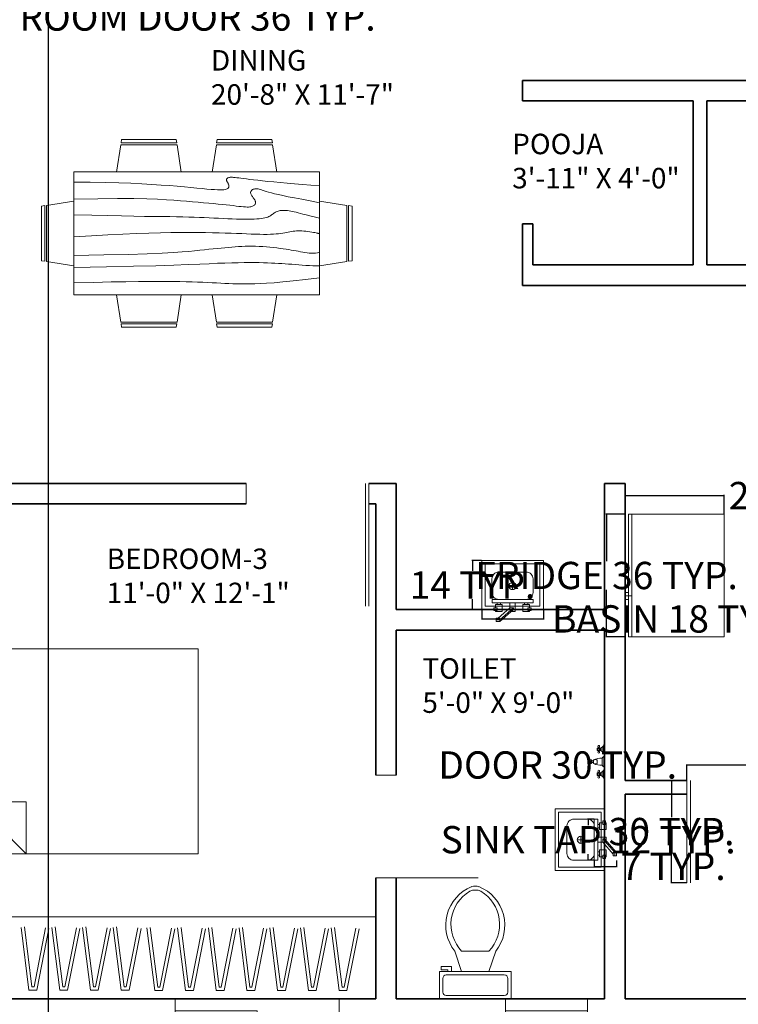
# Model space of a CAD drawing. Units: inches. Extents: x 3343 to 4790, y 1140 to 2641.
# Tile 4 of 10: x 3671 to 3881, y 2022 to 2310. Entities that reach past the tile are written whole.
import ezdxf

# ---------------------------------------------------------------- set-up
doc = ezdxf.new("R2010")
doc.units = ezdxf.units.IN
doc.header["$LTSCALE"] = 5
doc.header["$MEASUREMENT"] = 0
for name, color, linetype, lineweight in [('A-ANNO-DIMS', 2, 'Continuous', 18), ('A-AREA-IDEN', 7, 'Continuous', 18), ('A-DOOR', 3, 'Continuous', 18), ('A-EQPM', 9, 'Continuous', 18), ('A-FLOR-CASE', 9, 'Continuous', 18), ('A-FLOR-FIXT', 9, 'Continuous', 18), ('A-FURN', 8, 'Continuous', 13), ('A-GLAZ', 4, 'Continuous', 18), ('A-WALL', 7, 'Continuous', 35)]:
    doc.layers.add(name, color=color, linetype=linetype, lineweight=lineweight)
doc.styles.get("Standard").update_dxf_attribs({"font": 'arial.ttf'})
doc.dimstyles.get("Standard").update_dxf_attribs({"dimtxt": 8, "dimasz": 0.18, "dimexe": 0.18, "dimexo": 0.0625, "dimgap": 0.09, "dimtad": 0, "dimtih": 1, "dimtoh": 1, "dimdec": 1, "dimzin": 0, "dimdsep": 46, "dimlunit": 3, "dimtxsty": 'Standard', "dimcen": 0.09, "dimadec": 0, "dimazin": 0, "dimtfac": 1, "dimtdec": 1, "dimtofl": 0, "dimtmove": 0, "dimatfit": 3, "dimfxl": 1, "dimtolj": 1, "dimtzin": 0, "dimarcsym": 0})

# ---------------------------------------------------------------- blocks, each defined once
blk = doc.blocks.new('Bed - Queen')
for p, q in [((0, -80.00003), (0, 0)), ((0, 0), (59.99999, 0)), ((59.99999, 0), (59.99999, -80.00003)), ((7.99999, -1.2), (28.79998, -1.2)), ((7.99999, -14.4), (7.99999, -1.2)), ((28.79998, -1.2), (28.79998, -14.4)), ((31.19999, -1.2), (51.99999, -1.2)), ((31.19999, -14.4), (31.19999, -1.2)), ((51.99999, -1.2), (51.99999, -16.4)), ((0, -14.4), (44.8, -14.4)), ((59.99999, -29.6), (44.8, -14.4)), ((44.8, -14.4), (44.8, -29.6)), ((44.8, -16.8), (0, -16.8)), ((51.99999, -16.4), (46.79936, -16.4)), ((44.8, -29.6), (59.99999, -29.6)), ((59.99999, -80.00003), (0, -80.00003))]:
    blk.add_line(p, q)
blk = doc.blocks.new('Toilet - top')
for p, q in [((9.5, -6), (9.5, -2)), ((-10, -8.5), (-8, -8.5)), ((-10, -9.5), (-10, -8.5)), ((-8, -8.5), (-8, -8)), ((-7, -8), (-7, -9.5)), ((-4, -8), (-6, -14)), ((4, -8), (6, -14)), ((-7, -9.5), (-10, -9.5)), ((4, -14), (-4, -14))]:
    blk.add_line(p, q)
blk.add_lwpolyline([(10.5, -8), (10.5, 0), (-10.5, 0), (-10.5, -8)], close=True)
for points in [[(-9.5, -2), (-9.5, -6)], [(8.5, -1), (-8.5, -1)], [(-8.5, -7), (8.5, -7)]]:
    blk.add_lwpolyline(points)
for centre, radius, start, end in [((-8.62, -1.88), 0.884, 81.8699, 188.1301), ((8.62, -1.88), 0.884, 351.8699, 98.1301), ((-8.62, -6.12), 0.884, 171.8699, 278.1301), ((8.62, -6.12), 0.884, 261.8699, 8.1301), ((3.52, -21.58), 12.17, 141.4691, 247.9714), ((4.2, -21.82), 11.33, 136.3677, 238.9468), ((-3.52, -21.58), 12.17, 292.0284, 38.5307), ((-4.2, -21.82), 11.33, 301.053, 43.6321), ((0, -27.88), 4, 245.7318, 294.2682), ((0, -29), 4, 254.8605, 285.1395)]:
    blk.add_arc(centre, radius, start, end)
blk = doc.blocks.new('Faucet - Bathroom front')
for p, q in [((-0.5, 4.25), (0.5, 4.25)), ((0.5, 3.75), (-0.5, 3.75)), ((-0.5, 3), (0.5, 3)), ((-0.25, 3), (-0.25, 3.5)), ((0.25, 3.5), (0.25, 3)), ((-5, 0), (-2.25, 0)), ((-4.5087, 0.25), (-2.7408, 0.25)), ((-4, 1.625), (-4.25, 1.625)), ((-4, 1.375), (-4.25, 1.375)), ((-3.1442, 0.75), (-4.0979, 0.75)), ((-3.25, 1.625), (-3, 1.625)), ((-3.25, 1.375), (-3, 1.375)), ((-1.5, 0), (1.5, 0)), ((-1, 0.5), (1, 0.5)), ((0.5, 2), (-0.5, 2)), ((2.25, 0), (5, 0)), ((2.7413, 0.25), (4.5092, 0.25)), ((3.25, 1.625), (3, 1.625)), ((3.25, 1.375), (3, 1.375)), ((4.1058, 0.75), (3.1521, 0.75)), ((4, 1.625), (4.25, 1.625)), ((4, 1.375), (4.25, 1.375))]:
    blk.add_line(p, q)
for points in [[(-0.5, 3.75), (-0.5, 4.25)], [(-0.25, 4.5), (0.25, 4.5)], [(0.25, 3.5), (-0.25, 3.5)], [(0.5, 4.25), (0.5, 3.75)]]:
    blk.add_lwpolyline(points)
for points in [[(-4, 1), (-4, 2), (-3.25, 2), (-3.25, 1)], [(3.25, 1), (3.25, 2), (4, 2), (4, 1)]]:
    blk.add_lwpolyline(points, close=True)
for centre in [(-4.5, 1.5), (-3.625, 1.5), (-2.75, 1.5), (2.75, 1.5), (3.625, 1.5), (4.5, 1.5)]:
    blk.add_circle(centre, 0.2795)
for centre, radius, start, end in [((3, 1), 4.0311, 150.2551, 187.125), ((0.6413, 2.5), 1.246, 156.3417, 203.6583), ((-0.2575, 4.2575), 0.2426, 88.22243, 181.7776), ((-0.2575, 3.7425), 0.2426, 178.2224, 271.7776), ((0.2575, 4.2575), 0.2426, 358.2224, 91.77757), ((0.2575, 3.7425), 0.2426, 268.2224, 1.777565), ((-3, 1), 4.0311, 352.875, 29.74488), ((-0.6413, 2.5), 1.246, 336.3417, 23.65835), ((-5.375, 1.375), 1.4252, 285.2551, 344.7449), ((-1.875, 1.375), 1.4252, 195.2551, 254.7449), ((-0.7962, -0.2038), 0.7327, 106.1502, 163.8498), ((0.7962, -0.2038), 0.7327, 16.1502, 73.84979), ((1.875, 1.375), 1.4252, 285.2551, 344.7449), ((5.375, 1.375), 1.4252, 195.2551, 254.7449)]:
    blk.add_arc(centre, radius, start, end)
blk = doc.blocks.new('Faucet - kit sink front')
for p, q in [((-0.25, 3), (3.75, 6.5)), ((3.75, 6), (-0.25, 2.5)), ((3.75, 6), (3.75, 6.5)), ((3.75, 6.5), (4.75, 6.5)), ((3.75, 5.5), (3.75, 6)), ((4.75, 6), (3.75, 6)), ((4.75, 6.5), (4.75, 6)), ((4.75, 6), (4.75, 5.5)), ((-0.75, 3.5), (0.3192, 3.5)), ((-0.75, 1), (-0.75, 3.5)), ((-0.25, 2.5), (-0.25, 3)), ((4.1921, 5.5041), (0.75, 2.5)), ((4.75, 5.5), (3.75, 5.5)), ((-4.5, 1), (-4.5, 1.5)), ((-3.5, 1.5), (-3.5, 1)), ((0.75, 2.5), (-0.25, 2.5)), ((0.75, 2.5), (0.75, 1)), ((3.5, 1.5), (3.5, 1)), ((4.5, 1), (4.5, 1.5))]:
    blk.add_line(p, q)
for points in [[(-5.5, 2.5), (-5.5, 3.25), (-4.5, 3.25), (-4.5, 2.5)], [(5.5, 2.5), (5.5, 3.25), (4.5, 3.25), (4.5, 2.5)], [(-6, 0), (-6, 1), (6, 1), (6, 0)]]:
    blk.add_lwpolyline(points, close=True)
for points in [[(-5, 3.2513), (-5, 3.5), (-3, 3.5), (-3, 1.5), (-5, 1.5), (-5, 2.5)], [(5, 3.2513), (5, 3.5), (3, 3.5), (3, 1.5), (5, 1.5), (5, 2.5)]]:
    blk.add_lwpolyline(points)
blk = doc.blocks.new('Dining Set - 36 x 72 in.')
for p, q in [((-22.2343, 26.00059), (-23.4847, 17.99762)), ((-22.2304, 26), (-5.7608, 26)), ((-22, 27.5), (-22.1562, 26.50042)), ((-5.8416, 26.5), (-22.1534, 26.5)), ((-22, 27.5), (-6, 27.5)), ((-5.8437, 26.49966), (-6, 27.5)), ((-4.5152, 17.99762), (-5.7655, 25.99926)), ((5.7657, 26.00059), (4.5153, 17.99762)), ((5.7696, 26), (22.2392, 26)), ((6, 27.5), (5.8438, 26.50042)), ((22.1584, 26.5), (5.8466, 26.5)), ((6, 27.5), (22, 27.5)), ((22.1563, 26.49966), (22, 27.5)), ((23.4848, 17.99762), (22.2345, 25.99926)), ((36, 18), (-36, 18)), ((-36, 18), (-36, -18)), ((36, -18), (36, 18)), ((-44.0006, 8.23428), (-35.9976, 9.48474)), ((44.0006, 8.23428), (35.9976, 9.48474)), ((-45.5, 8), (-44.5004, 8.15617)), ((-45.5, 8), (-45.5, -8)), ((-44.5, -8.15843), (-44.5, 8.15338)), ((-44, 8.23041), (-44, -8.23915)), ((44, 8.23041), (44, -8.23915)), ((44.5, -8.15843), (44.5, 8.15338)), ((45.5, 8), (44.5005, 8.15617)), ((45.5, 8), (45.5, -8)), ((-44.4997, -8.15631), (-45.5, -8)), ((-35.9976, -9.48476), (-43.9993, -8.2345)), ((35.9976, -9.48476), (43.9993, -8.2345)), ((44.4997, -8.15631), (45.5, -8)), ((-36, -18), (36, -18)), ((-22.2343, -26.0006), (-23.4847, -17.99762)), ((-4.5152, -17.99762), (-5.7655, -25.99928)), ((5.7657, -26.0006), (4.5153, -17.99762)), ((23.4848, -17.99762), (22.2345, -25.99928)), ((-22.2304, -26), (-5.7608, -26)), ((-22, -27.5), (-22.1562, -26.50044)), ((-5.8416, -26.5), (-22.1534, -26.5)), ((-22, -27.5), (-6, -27.5)), ((-5.8437, -26.49967), (-6, -27.5)), ((5.7696, -26), (22.2392, -26)), ((6, -27.5), (5.8438, -26.50044)), ((22.1584, -26.5), (5.8466, -26.5)), ((6, -27.5), (22, -27.5)), ((22.1563, -26.49967), (22, -27.5))]:
    blk.add_line(p, q)
for points in [[(-36, 15), (-31.1772, 14.97754), (-26.8079, 14.91406), (-22.8538, 14.81543), (-19.276, 14.6875), (-16.0362, 14.53613), (-13.0957, 14.36718), (-10.4159, 14.18652), (-7.9583, 14), (-5.6904, 13.81315), (-3.6035, 13.63021), (-1.6954, 13.45508), (0.0365, 13.29166), (1.5945, 13.14388), (2.9811, 13.01562), (4.1988, 12.9108), (5.25, 12.83333), (6.1393, 12.78613), (6.8802, 12.76823), (7.4883, 12.77767), (7.9792, 12.8125), (8.3685, 12.87077), (8.6719, 12.95052), (8.9049, 13.0498), (9.0833, 13.16666), (9.2205, 13.29899), (9.3216, 13.44401), (9.3895, 13.59879), (9.4271, 13.76041), (9.4373, 13.92594), (9.4232, 14.09245), (9.3875, 14.257), (9.3333, 14.41666), (9.2638, 14.56917), (9.1836, 14.71484), (9.0975, 14.85465), (9.0104, 14.98958), (8.9272, 15.1206), (8.8529, 15.2487), (8.7922, 15.37483), (8.75, 15.5), (8.7305, 15.62467), (8.7344, 15.74739), (8.7617, 15.86621), (8.8125, 15.97916), (8.8867, 16.08431), (8.9844, 16.17968), (9.1055, 16.26334), (9.25, 16.33333), (9.4189, 16.38802), (9.6172, 16.42708), (9.8506, 16.45052), (10.125, 16.45833), (10.4463, 16.45052), (10.8203, 16.42708), (11.2529, 16.38802), (11.75, 16.33333), (12.3184, 16.26318), (12.9694, 16.17838), (13.7151, 16.07991), (14.5677, 15.96875), (15.5395, 15.84586), (16.6426, 15.71224), (17.8893, 15.56884), (19.2917, 15.41666), (20.859, 15.25667), (22.5879, 15.08984), (24.4721, 14.91715), (26.5052, 14.73958), (28.6809, 14.5581), (30.9929, 14.3737), (33.4347, 14.18733), (36, 14)], [(-36, 10), (-28.9766, 10.14274), (-23.1725, 10.20442), (-18.4241, 10.19775), (-14.5677, 10.13541), (-11.4399, 10.03011), (-8.877, 9.89453), (-6.7154, 9.74137), (-4.7917, 9.58333), (-2.9698, 9.43082), (-1.2246, 9.28515), (0.4415, 9.14534), (2.026, 9.01041), (3.5266, 8.87939), (4.9408, 8.7513), (6.266, 8.62516), (7.5, 8.5), (8.6411, 8.37549), (9.6914, 8.2539), (10.6538, 8.13818), (11.5312, 8.03125), (12.3267, 7.93603), (13.043, 7.85547), (13.6831, 7.79248), (14.25, 7.75), (14.7471, 7.7303), (15.1797, 7.73307), (15.5537, 7.75732), (15.875, 7.80208), (16.1494, 7.86637), (16.3828, 7.94922), (16.5811, 8.04964), (16.75, 8.16666), (16.8944, 8.29915), (17.0143, 8.44531), (17.1089, 8.60319), (17.1771, 8.77083), (17.218, 8.94629), (17.2305, 9.1276), (17.2137, 9.31282), (17.1667, 9.5), (17.0895, 9.6875), (16.987, 9.875), (16.8649, 10.0625), (16.7292, 10.25), (16.5856, 10.4375), (16.4401, 10.625), (16.2985, 10.8125), (16.1667, 11), (16.05, 11.18733), (15.9518, 11.3737), (15.8752, 11.5581), (15.8229, 11.73958), (15.798, 11.91715), (15.8034, 12.08984), (15.842, 12.25667), (15.9167, 12.41666), (16.0295, 12.56836), (16.1784, 12.70833), (16.3605, 12.83268), (16.5729, 12.9375), (16.8127, 13.01888), (17.0768, 13.07291), (17.3625, 13.0957), (17.6667, 13.08333), (17.9894, 13.03312), (18.3418, 12.94726), (18.7382, 12.82918), (19.1927, 12.68229), (19.7195, 12.51001), (20.3327, 12.31575), (21.0465, 12.10294), (21.875, 11.875), (22.8357, 11.63354), (23.959, 11.37304), (25.2786, 11.08618), (26.8282, 10.76562), (28.6414, 10.40405), (30.752, 9.99414), (33.1936, 9.52856), (36, 9)], [(-36, 5.5), (-30.7157, 5.3348), (-26.069, 5.20963), (-21.9946, 5.11767), (-18.4271, 5.05208), (-15.3009, 5.00602), (-12.5508, 4.97265), (-10.1112, 4.94515), (-7.9167, 4.91666), (-5.909, 4.88167), (-4.0586, 4.83984), (-2.3429, 4.79215), (-0.7396, 4.73958), (0.7739, 4.6831), (2.22, 4.6237), (3.6213, 4.56233), (5, 4.5), (6.373, 4.43782), (7.7344, 4.3776), (9.0723, 4.32129), (10.375, 4.27083), (11.6309, 4.22819), (12.8281, 4.19531), (13.9551, 4.17415), (15, 4.16666), (15.954, 4.17448), (16.819, 4.19791), (17.6001, 4.23698), (18.3021, 4.29166), (18.9299, 4.36198), (19.4883, 4.44791), (19.9823, 4.54948), (20.4167, 4.66666), (20.7969, 4.79899), (21.1302, 4.94401), (21.4245, 5.09879), (21.6875, 5.26041), (21.9271, 5.42594), (22.1511, 5.59245), (22.3672, 5.757), (22.5834, 5.91666), (22.8065, 6.06868), (23.0404, 6.21093), (23.2879, 6.34147), (23.5521, 6.45833), (23.8358, 6.55957), (24.142, 6.64323), (24.4735, 6.70735), (24.8334, 6.75), (25.2235, 6.76969), (25.642, 6.76692), (26.0858, 6.74267), (26.5521, 6.69791), (27.0379, 6.63362), (27.5404, 6.55078), (28.0565, 6.45036), (28.5834, 6.33333), (29.1242, 6.19987), (29.7071, 6.04687), (30.3661, 5.87044), (31.1354, 5.66666), (32.0493, 5.43164), (33.142, 5.16146), (34.4475, 4.85221), (36, 4.5)], [(-36, -1), (-30.7915, -0.6591), (-26.0195, -0.38216), (-21.6519, -0.16284), (-17.6563, 0.00521), (-14.0005, 0.12833), (-10.6523, 0.21289), (-7.5796, 0.26522), (-4.75, 0.29166), (-2.134, 0.29793), (0.2878, 0.28711), (2.5317, 0.26163), (4.6146, 0.22396), (6.5529, 0.17651), (8.3633, 0.12174), (10.0623, 0.06209), (11.6667, 0), (13.1899, -0.06201), (14.6341, -0.1211), (15.9982, -0.17432), (17.2813, -0.21875), (18.4823, -0.25147), (19.6003, -0.26953), (20.6343, -0.27002), (21.5834, -0.25), (22.4481, -0.20768), (23.2357, -0.14584), (23.9549, -0.06836), (24.6146, 0.02083), (25.2235, 0.11784), (25.7904, 0.21875), (26.3241, 0.31966), (26.8334, 0.41666), (27.3265, 0.50618), (27.8099, 0.58593), (28.2894, 0.65397), (28.7709, 0.70833), (29.2601, 0.74707), (29.763, 0.76823), (30.2855, 0.76985), (30.8334, 0.75), (31.4088, 0.70784), (31.9994, 0.64713), (32.589, 0.57275), (33.1615, 0.48958), (33.7008, 0.4025), (34.1908, 0.3164), (34.6153, 0.23616), (34.9584, 0.16666), (35.2099, 0.11165), (35.3848, 0.07031), (35.504, 0.04069), (35.5886, 0.02083), (35.6594, 0.00879), (35.7377, 0.0026), (35.8442, 0.00032), (36, 0)], [(-36, -6.5), (-27.1843, -6.31267), (-20.084, -6.1263), (-14.469, -5.9419), (-10.1094, -5.76042), (-6.7752, -5.58285), (-4.2363, -5.41016), (-2.2629, -5.24333), (-0.625, -5.08334), (0.8708, -4.93099), (2.2715, -4.78646), (3.5872, -4.64974), (4.8281, -4.52084), (6.0046, -4.39974), (7.127, -4.28646), (8.2053, -4.18099), (9.25, -4.08334), (10.2705, -3.99382), (11.2734, -3.91407), (12.2647, -3.84603), (13.25, -3.79167), (14.2354, -3.75293), (15.2266, -3.73177), (16.2295, -3.73015), (17.25, -3.75), (18.2912, -3.79248), (19.3451, -3.85547), (20.4009, -3.93604), (21.4479, -4.03125), (22.4754, -4.13819), (23.4727, -4.25391), (24.4289, -4.37549), (25.3334, -4.5), (26.1785, -4.62492), (26.9694, -4.74935), (27.7145, -4.87281), (28.4219, -4.99479), (29.1, -5.11483), (29.7572, -5.23242), (30.4016, -5.34709), (31.0417, -5.45834), (31.6837, -5.56437), (32.3262, -5.65821), (32.9658, -5.73153), (33.599, -5.77604), (34.2224, -5.78345), (34.8327, -5.74545), (35.4264, -5.65373), (36, -5.5)], [(-36, -10), (-26.4022, -9.81299), (-18.4675, -9.62891), (-11.9839, -9.45069), (-6.7396, -9.28125), (-2.5226, -9.12354), (0.8789, -8.98047), (3.6769, -8.85498), (6.0833, -8.75), (8.2767, -8.66765), (10.3021, -8.60677), (12.1712, -8.56543), (13.8958, -8.54167), (15.4876, -8.53353), (16.9583, -8.53907), (18.3197, -8.55632), (19.5834, -8.58334), (20.7616, -8.61841), (21.8685, -8.66081), (22.9188, -8.71004), (23.9271, -8.76563), (24.9081, -8.82707), (25.8763, -8.89388), (26.8465, -8.96558), (27.8334, -9.04167), (28.8474, -9.12118), (29.8828, -9.20117), (30.93, -9.27824), (31.9792, -9.34896), (33.0205, -9.40991), (34.0443, -9.45768), (35.0407, -9.48885), (36, -9.5)], [(-36, -14.5), (-30.0881, -14.33513), (-25.0332, -14.21224), (-20.7312, -14.12647), (-17.0781, -14.07292), (-13.97, -14.04671), (-11.3027, -14.04297), (-8.9724, -14.05681), (-6.875, -14.08334), (-4.9224, -14.11833), (-3.0905, -14.16016), (-1.3709, -14.20785), (0.2448, -14.26042), (1.7647, -14.3169), (3.1973, -14.3763), (4.5507, -14.43767), (5.8333, -14.5), (7.0554, -14.5621), (8.235, -14.62175), (9.3922, -14.67652), (10.5469, -14.72396), (11.7192, -14.76164), (12.929, -14.78711), (14.1965, -14.79794), (15.5417, -14.79167), (16.9933, -14.76424), (18.6152, -14.70508), (20.4804, -14.60197), (22.6615, -14.44271), (25.2312, -14.21509), (28.2624, -13.9069), (31.8277, -13.50594), (36, -13)]]:
    blk.add_lwpolyline(points)
blk = doc.blocks.new('Refrigerator-2 door - 36 in top')
for p, q in [((0, -26.999999), (36, -26.999999)), ((11, -27.999999), (11, -28.999999)), ((12, -26.999999), (12, -28.999999)), ((13, -28.999999), (13, -27.999999)), ((11, -28.999999), (13, -28.999999))]:
    blk.add_line(p, q)
blk.add_lwpolyline([(0, -27.999999), (0, 0), (36, 0), (36, -27.999999)], close=True)
blk = doc.blocks.new('SINK-BOWL-WITH-DRAIN')
for p, q in [((8.58, 9.03), (6.47, 9.03)), ((7.52, 10.09), (7.52, 7.97))]:
    blk.add_line(p, q)
for points in [[(14.44, 0), (0, 0), (0, 18.06), (14.44, 18.06)], [(1, 1), (1, 17.06), (13.44, 17.06), (13.44, 1)]]:
    blk.add_lwpolyline(points, close=True)
blk.add_lwpolyline([(9.44, 15.06), (5.44, 15.06, 0.414214), (3.44, 13.06), (3.44, 5, 0.414214), (5.44, 3), (9.44, 3, 0.414214), (11.44, 5), (11.44, 13.06, 0.414214)], format="xyb", close=True)
blk.add_circle((7.52, 9.03), 1.06)
blk = doc.blocks.new('WINDOW-48IN-SLIDING-JAMB9')
for p, q in [((0, 9), (0, 0)), ((48, 9), (48, 0)), ((0, 5.5), (24, 5.5)), ((0, 4.5), (48, 4.5)), ((24, 5.5), (24, 3.5)), ((24, 3.5), (48, 3.5))]:
    blk.add_line(p, q)
blk = doc.blocks.new('WINDOW-24IN-FIXED')
for p, q in [((0, 9), (0, 0)), ((24, 9), (24, 0)), ((0, 5.5), (24, 5.5)), ((0, 3.5), (24, 3.5))]:
    blk.add_line(p, q)
blk = doc.blocks.new('DOOR-36IN-6IN-JAMB-DBL-LINE')
at = {"ltscale": 5}
for p, q in [((35, 0), (35, 36)), ((36, 0), (36, 36)), ((0, 6), (0, 0)), ((36, 6), (36, 0))]:
    blk.add_line(p, q, dxfattribs=at)
blk = doc.blocks.new('DOOR-30IN-4IN-JAMB-DBL-LINE')
at = {"ltscale": 5}
for p, q in [((29, 0), (29, 30)), ((30, 0), (30, 30)), ((0, 4), (0, 0)), ((30, 4), (30, 0))]:
    blk.add_line(p, q, dxfattribs=at)
blk = doc.blocks.new('WARDROBE-HANGER')
for points in [[(0.22, 7.19), (17.51, 3.78), (17.51, 3.18), (0, 0.99)], [(0.41, 8.17), (18.51, 4.61), (18.51, 2.3), (0.12, 0)]]:
    blk.add_lwpolyline(points)
blk = doc.blocks.new('*D33')
at = {"layer": 'A-ANNO-DIMS', "color": 0, "lineweight": -2, "ltscale": 5, "transparency": 16777216}
for p, q in [((3839.07, 2075.77), (3837.15, 2075.77)), ((3837.33, 2075.59), (3837.33, 2073.99)), ((3837.33, 2063.95), (3837.33, 2065.54)), ((3839.07, 2063.77), (3837.15, 2063.77))]:
    blk.add_line(p, q, dxfattribs=at)
at = {"layer": 'A-ANNO-DIMS', "color": 0, "ltscale": 5, "transparency": 16777216}
for points in [[(3837.3, 2075.59), (3837.36, 2075.59), (3837.33, 2075.77)], [(3837.3, 2063.95), (3837.36, 2063.95), (3837.33, 2063.77)]]:
    blk.add_solid(points, dxfattribs=at)
at = {"layer": 'Defpoints', "color": 0, "ltscale": 5, "transparency": 16777216}
for p in [(3839.13, 2075.77), (3837.33, 2063.77), (3839.13, 2063.77)]:
    blk.add_point(p, dxfattribs=at)
at = {"layer": 'A-ANNO-DIMS', "color": 0, "ltscale": 5, "transparency": 16777216, "insert": (3837.33, 2069.77), "char_height": 8, "attachment_point": 5}
blk.add_mtext('\\A1;SINK TAP 12 TYP.', dxfattribs=at)
blk = doc.blocks.new('*D34')
at = {"layer": 'A-ANNO-DIMS', "color": 0, "lineweight": -2, "ltscale": 5, "transparency": 16777216}
for p, q in [((3839.13, 2063.7), (3839.13, 2061.79)), ((3845.63, 2063.7), (3845.63, 2061.79)), ((3839.31, 2061.97), (3845.45, 2061.97)), ((3845.63, 2061.97), (3845.81, 2061.97))]:
    blk.add_line(p, q, dxfattribs=at)
at = {"layer": 'A-ANNO-DIMS', "color": 0, "ltscale": 5, "transparency": 16777216}
for points in [[(3839.31, 2062), (3839.31, 2061.94), (3839.13, 2061.97)], [(3845.45, 2062), (3845.45, 2061.94), (3845.63, 2061.97)]]:
    blk.add_solid(points, dxfattribs=at)
at = {"layer": 'Defpoints', "color": 0, "ltscale": 5, "transparency": 16777216}
for p in [(3839.13, 2063.77), (3845.63, 2063.77), (3845.63, 2061.97)]:
    blk.add_point(p, dxfattribs=at)
at = {"layer": 'A-ANNO-DIMS', "color": 0, "ltscale": 5, "transparency": 16777216, "insert": (3862.23, 2061.97), "char_height": 8, "attachment_point": 5}
blk.add_mtext('\\A1;7 TYP.', dxfattribs=at)
blk = doc.blocks.new('*D51')
at = {"layer": 'A-ANNO-DIMS', "color": 0, "lineweight": -2, "ltscale": 5, "transparency": 16777216}
for p, q in [((3806.15, 2137.1), (3806.15, 2134.27)), ((3824.22, 2137.1), (3824.22, 2134.27)), ((3806.33, 2134.45), (3824.04, 2134.45)), ((3824.22, 2134.45), (3824.4, 2134.45))]:
    blk.add_line(p, q, dxfattribs=at)
at = {"layer": 'A-ANNO-DIMS', "color": 0, "ltscale": 5, "transparency": 16777216}
for points in [[(3806.33, 2134.48), (3806.33, 2134.42), (3806.15, 2134.45)], [(3824.04, 2134.48), (3824.04, 2134.42), (3824.22, 2134.45)]]:
    blk.add_solid(points, dxfattribs=at)
at = {"layer": 'Defpoints', "color": 0, "ltscale": 5, "transparency": 16777216}
for p in [(3806.15, 2137.16), (3824.22, 2137.16), (3824.22, 2134.45)]:
    blk.add_point(p, dxfattribs=at)
at = {"layer": 'A-ANNO-DIMS', "color": 0, "ltscale": 5, "transparency": 16777216, "insert": (3862.1, 2134.45), "char_height": 8, "attachment_point": 5}
blk.add_mtext('\\A1;BASIN 18 TYP.', dxfattribs=at)
blk = doc.blocks.new('*D52')
at = {"layer": 'A-ANNO-DIMS', "color": 0, "lineweight": -2, "ltscale": 5, "transparency": 16777216}
for p, q in [((3806.09, 2151.6), (3803.27, 2151.6)), ((3803.45, 2151.42), (3803.45, 2148.49)), ((3803.45, 2137.34), (3803.45, 2140.27)), ((3806.09, 2137.16), (3803.27, 2137.16))]:
    blk.add_line(p, q, dxfattribs=at)
at = {"layer": 'A-ANNO-DIMS', "color": 0, "ltscale": 5, "transparency": 16777216}
for points in [[(3803.42, 2151.42), (3803.48, 2151.42), (3803.45, 2151.6)], [(3803.42, 2137.34), (3803.48, 2137.34), (3803.45, 2137.16)]]:
    blk.add_solid(points, dxfattribs=at)
at = {"layer": 'Defpoints', "color": 0, "ltscale": 5, "transparency": 16777216}
for p in [(3806.15, 2151.6), (3803.45, 2137.16), (3806.15, 2137.16)]:
    blk.add_point(p, dxfattribs=at)
at = {"layer": 'A-ANNO-DIMS', "color": 0, "ltscale": 5, "transparency": 16777216, "insert": (3803.45, 2144.38), "char_height": 8, "attachment_point": 5}
blk.add_mtext('\\A1;14 TYP.', dxfattribs=at)
blk = doc.blocks.new('*D65')
at = {"layer": 'A-ANNO-DIMS', "color": 0, "lineweight": -2, "ltscale": 5, "transparency": 16777216}
for p, q in [((3630.13, 2316.1), (3630.13, 2310.58)), ((3666.13, 2316.1), (3666.13, 2310.58)), ((3630.31, 2310.76), (3665.95, 2310.76)), ((3666.13, 2310.76), (3666.31, 2310.76))]:
    blk.add_line(p, q, dxfattribs=at)
at = {"layer": 'A-ANNO-DIMS', "color": 0, "ltscale": 5, "transparency": 16777216}
for points in [[(3630.31, 2310.79), (3630.31, 2310.73), (3630.13, 2310.76)], [(3665.95, 2310.79), (3665.95, 2310.73), (3666.13, 2310.76)]]:
    blk.add_solid(points, dxfattribs=at)
at = {"layer": 'Defpoints', "color": 0, "ltscale": 5, "transparency": 16777216}
for p in [(3630.13, 2316.16), (3666.13, 2316.16), (3666.13, 2310.76)]:
    blk.add_point(p, dxfattribs=at)
at = {"layer": 'A-ANNO-DIMS', "color": 0, "ltscale": 5, "transparency": 16777216, "insert": (3722.92, 2310.76), "char_height": 8, "attachment_point": 5}
blk.add_mtext('\\A1;ROOM DOOR 36 TYP.', dxfattribs=at)
blk = doc.blocks.new('*D71')
at = {"layer": 'A-ANNO-DIMS', "color": 0, "lineweight": -2, "ltscale": 5, "transparency": 16777216}
for p, q in [((3848.07, 2165.17), (3842.55, 2165.17)), ((3842.73, 2164.99), (3842.73, 2151.4)), ((3842.73, 2129.35), (3842.73, 2142.94)), ((3848.07, 2129.17), (3842.55, 2129.17))]:
    blk.add_line(p, q, dxfattribs=at)
at = {"layer": 'A-ANNO-DIMS', "color": 0, "ltscale": 5, "transparency": 16777216}
for points in [[(3842.7, 2164.99), (3842.76, 2164.99), (3842.73, 2165.17)], [(3842.7, 2129.35), (3842.76, 2129.35), (3842.73, 2129.17)]]:
    blk.add_solid(points, dxfattribs=at)
at = {"layer": 'Defpoints', "color": 0, "ltscale": 5, "transparency": 16777216}
for p in [(3842.73, 2165.17), (3848.13, 2165.17), (3848.13, 2129.17)]:
    blk.add_point(p, dxfattribs=at)
at = {"layer": 'A-ANNO-DIMS', "color": 0, "ltscale": 5, "transparency": 16777216, "insert": (3842.73, 2147.17), "char_height": 8, "attachment_point": 5}
blk.add_mtext('\\A1;FRIDGE 36 TYP.', dxfattribs=at)
blk = doc.blocks.new('*D72')
at = {"layer": 'A-ANNO-DIMS', "color": 0, "lineweight": -2, "ltscale": 5, "transparency": 16777216}
for p, q in [((3848.13, 2165.23), (3848.13, 2170.75)), ((3848.31, 2170.57), (3876.95, 2170.57)), ((3877.13, 2165.23), (3877.13, 2170.75)), ((3877.13, 2170.57), (3877.31, 2170.57))]:
    blk.add_line(p, q, dxfattribs=at)
at = {"layer": 'A-ANNO-DIMS', "color": 0, "ltscale": 5, "transparency": 16777216}
for points in [[(3848.31, 2170.6), (3848.31, 2170.54), (3848.13, 2170.57)], [(3876.95, 2170.6), (3876.95, 2170.54), (3877.13, 2170.57)]]:
    blk.add_solid(points, dxfattribs=at)
at = {"layer": 'Defpoints', "color": 0, "ltscale": 5, "transparency": 16777216}
for p in [(3877.13, 2170.57), (3848.13, 2165.17), (3877.13, 2165.17)]:
    blk.add_point(p, dxfattribs=at)
at = {"layer": 'A-ANNO-DIMS', "color": 0, "ltscale": 5, "transparency": 16777216, "insert": (3896.94, 2170.57), "char_height": 8, "attachment_point": 5}
blk.add_mtext('\\A1;29 TYP.', dxfattribs=at)
blk = doc.blocks.new('*D81')
at = {"layer": 'A-ANNO-DIMS', "color": 0, "lineweight": -2, "ltscale": 5, "transparency": 16777216}
for p, q in [((3866.27, 2091.66), (3866.09, 2091.66)), ((3866.27, 2087.22), (3866.27, 2091.84)), ((3896.09, 2091.66), (3866.45, 2091.66)), ((3896.27, 2087.22), (3896.27, 2091.84))]:
    blk.add_line(p, q, dxfattribs=at)
at = {"layer": 'A-ANNO-DIMS', "color": 0, "ltscale": 5, "transparency": 16777216}
for points in [[(3866.45, 2091.69), (3866.45, 2091.63), (3866.27, 2091.66)], [(3896.09, 2091.69), (3896.09, 2091.63), (3896.27, 2091.66)]]:
    blk.add_solid(points, dxfattribs=at)
at = {"layer": 'Defpoints', "color": 0, "ltscale": 5, "transparency": 16777216}
for p in [(3866.27, 2091.66), (3866.27, 2087.16), (3896.27, 2087.16)]:
    blk.add_point(p, dxfattribs=at)
at = {"layer": 'A-ANNO-DIMS', "color": 0, "ltscale": 5, "transparency": 16777216, "insert": (3828.41, 2091.66), "char_height": 8, "attachment_point": 5}
blk.add_mtext('\\A1;DOOR 30 TYP.', dxfattribs=at)
blk = doc.blocks.new('*D82')
at = {"layer": 'A-ANNO-DIMS', "color": 0, "lineweight": -2, "ltscale": 5, "transparency": 16777216}
for p, q in [((3866.2, 2087.16), (3861.59, 2087.16)), ((3861.77, 2086.98), (3861.77, 2076.34)), ((3861.77, 2057.34), (3861.77, 2067.98)), ((3866.2, 2057.16), (3861.59, 2057.16))]:
    blk.add_line(p, q, dxfattribs=at)
at = {"layer": 'A-ANNO-DIMS', "color": 0, "ltscale": 5, "transparency": 16777216}
for points in [[(3861.74, 2086.98), (3861.8, 2086.98), (3861.77, 2087.16)], [(3861.74, 2057.34), (3861.8, 2057.34), (3861.77, 2057.16)]]:
    blk.add_solid(points, dxfattribs=at)
at = {"layer": 'Defpoints', "color": 0, "ltscale": 5, "transparency": 16777216}
for p in [(3866.27, 2087.16), (3861.77, 2057.16), (3866.27, 2057.16)]:
    blk.add_point(p, dxfattribs=at)
at = {"layer": 'A-ANNO-DIMS', "color": 0, "ltscale": 5, "transparency": 16777216, "insert": (3861.77, 2072.16), "char_height": 8, "attachment_point": 5}
blk.add_mtext('\\A1;30 TYP.', dxfattribs=at)
blk = doc.blocks.new('*D83')
at = {"layer": 'A-ANNO-DIMS', "color": 0, "lineweight": -2, "ltscale": 5, "transparency": 16777216}
for p, q in [((3424.13, 2432.05), (3424.13, 2635.49)), ((3424.31, 2635.31), (4052.48, 2635.31)), ((4703.95, 2635.31), (4075.77, 2635.31)), ((4704.13, 2197.22), (4704.13, 2635.49))]:
    blk.add_line(p, q, dxfattribs=at)
at = {"layer": 'A-ANNO-DIMS', "color": 0, "ltscale": 5, "transparency": 16777216}
for points in [[(3424.31, 2635.34), (3424.31, 2635.28), (3424.13, 2635.31)], [(4703.95, 2635.34), (4703.95, 2635.28), (4704.13, 2635.31)]]:
    blk.add_solid(points, dxfattribs=at)
at = {"layer": 'Defpoints', "color": 0, "ltscale": 5, "transparency": 16777216}
for p in [(4704.13, 2635.31), (3424.13, 2431.99), (4704.13, 2197.16)]:
    blk.add_point(p, dxfattribs=at)
at = {"layer": 'A-ANNO-DIMS', "color": 0, "ltscale": 5, "transparency": 16777216, "insert": (4064.13, 2635.31), "char_height": 8, "attachment_point": 5}
blk.add_mtext('\\A1;1280', dxfattribs=at)
blk = doc.blocks.new('*D84')
at = {"layer": 'A-ANNO-DIMS', "color": 0, "lineweight": -2, "ltscale": 5, "transparency": 16777216}
for p, q in [((3448.07, 2566.16), (3354.8, 2566.16)), ((3354.98, 2565.98), (3354.98, 1894.31)), ((3354.98, 1214.29), (3354.98, 1885.96)), ((4015.58, 1214.11), (3354.8, 1214.11))]:
    blk.add_line(p, q, dxfattribs=at)
at = {"layer": 'A-ANNO-DIMS', "color": 0, "ltscale": 5, "transparency": 16777216}
for points in [[(3354.95, 2565.98), (3355.01, 2565.98), (3354.98, 2566.16)], [(3354.95, 1214.29), (3355.01, 1214.29), (3354.98, 1214.11)]]:
    blk.add_solid(points, dxfattribs=at)
at = {"layer": 'Defpoints', "color": 0, "ltscale": 5, "transparency": 16777216}
for p in [(3448.13, 2566.16), (3354.98, 1214.11), (4015.65, 1214.11)]:
    blk.add_point(p, dxfattribs=at)
at = {"layer": 'A-ANNO-DIMS', "color": 0, "ltscale": 5, "transparency": 16777216, "insert": (3354.98, 1890.14), "char_height": 8, "attachment_point": 5}
blk.add_mtext('\\A1;1352', dxfattribs=at)
blk = doc.blocks.new('*D96')
at = {"layer": 'A-ANNO-DIMS', "color": 0, "lineweight": -2, "ltscale": 5, "transparency": 16777216}
for p, q in [((3619.25, 1835.73), (3619.25, 2635.49)), ((3619.43, 2635.31), (3643.42, 2635.31)), ((3679.07, 2635.31), (3655.08, 2635.31)), ((3679.25, 1835.73), (3679.25, 2635.49))]:
    blk.add_line(p, q, dxfattribs=at)
at = {"layer": 'A-ANNO-DIMS', "color": 0, "ltscale": 5, "transparency": 16777216}
for points in [[(3619.43, 2635.34), (3619.43, 2635.28), (3619.25, 2635.31)], [(3679.07, 2635.34), (3679.07, 2635.28), (3679.25, 2635.31)]]:
    blk.add_solid(points, dxfattribs=at)
at = {"layer": 'Defpoints', "color": 0, "ltscale": 5, "transparency": 16777216}
for p in [(3679.25, 2635.31), (3619.25, 1835.67), (3679.25, 1835.67)]:
    blk.add_point(p, dxfattribs=at)
at = {"layer": 'A-ANNO-DIMS', "color": 0, "ltscale": 5, "transparency": 16777216, "insert": (3649.25, 2635.31), "char_height": 8, "attachment_point": 5}
blk.add_mtext('\\A1;60', dxfattribs=at)

msp = doc.modelspace()

# ---------------------------------------------------------------- linework, layer by layer
at = {"layer": 'A-DOOR', "ltscale": 5}
for p, q in [((3775.13, 2088.654), (3781.13, 2088.654)), ((3775.13, 2058.654), (3781.13, 2058.654)), ((3775.13, 2058.654), (3805.13, 2058.654))]:
    msp.add_line(p, q, dxfattribs=at)
at = {"layer": 'A-FLOR-CASE', "ltscale": 5}
msp.add_line((3775.13, 2047.161), (3643.13, 2047.161), dxfattribs=at)
at = {"layer": 'A-FLOR-FIXT'}
for p, q in [((3835.218, 2070.827), (3835.218, 2068.708)), ((3836.277, 2069.767), (3834.158, 2069.767))]:
    msp.add_line(p, q, dxfattribs=at)
for points in [[(3842.13, 2060.736), (3827.693, 2060.736), (3827.693, 2078.799), (3842.13, 2078.799)], [(3828.693, 2061.736), (3828.693, 2077.799), (3841.13, 2077.799), (3841.13, 2061.736)]]:
    msp.add_lwpolyline(points, close=True, dxfattribs=at)
msp.add_lwpolyline([(3837.13, 2075.799), (3833.13, 2075.799, 0.4142136), (3831.13, 2073.799), (3831.13, 2065.736, 0.4142136), (3833.13, 2063.736), (3837.13, 2063.736, 0.4142136), (3839.13, 2065.736), (3839.13, 2073.799, 0.4142136)], format="xyb", close=True, dxfattribs=at)
msp.add_circle((3835.218, 2069.767), 1.06, dxfattribs=at)
at = {"layer": 'A-WALL', "ltscale": 5}
for p, q in [((3818.13, 2292.161), (3818.13, 2286.161)), ((3894.654, 2292.161), (3818.13, 2292.161)), ((3821.13, 2286.161), (3818.13, 2286.161)), ((3868.13, 2286.161), (3821.13, 2286.161)), ((3894.654, 2286.161), (3872.13, 2286.161)), ((3821.13, 2250.161), (3818.13, 2250.161)), ((3818.13, 2250.161), (3818.13, 2232.161)), ((3868.13, 2238.161), (3821.13, 2238.161)), ((3907.995, 2238.161), (3872.13, 2238.161)), ((3907.995, 2232.161), (3818.13, 2232.161)), ((3737.13, 2174.161), (3635.13, 2174.161)), ((3781.13, 2174.161), (3773.13, 2174.161)), ((3842.13, 2174.161), (3848.13, 2174.161)), ((3737.13, 2168.161), (3643.13, 2168.161)), ((3775.13, 2168.161), (3773.13, 2168.161)), ((3842.13, 2137.161), (3781.13, 2137.161)), ((3842.13, 2131.161), (3781.13, 2131.161)), ((3866.266, 2087.161), (3848.13, 2087.161)), ((3866.266, 2083.161), (3848.13, 2083.161)), ((3775.13, 2023.161), (3643.13, 2023.161)), ((3842.13, 2023.161), (3781.13, 2023.161)), ((3968.13, 2023.161), (3848.13, 2023.161))]:
    msp.add_line(p, q, dxfattribs=at)
at = {"layer": 'A-WALL'}
for p, q in [((3868.13, 2286.161), (3868.13, 2238.161)), ((3872.13, 2286.161), (3872.13, 2238.161)), ((3821.13, 2250.161), (3821.13, 2238.161)), ((3781.13, 2174.161), (3781.13, 2137.161)), ((3842.13, 2174.161), (3842.13, 2137.161)), ((3848.13, 2174.161), (3848.13, 2087.161)), ((3775.13, 2168.161), (3775.13, 2088.654)), ((3781.13, 2131.161), (3781.13, 2088.654)), ((3842.13, 2131.161), (3842.13, 2023.161)), ((3842.13, 2083.161), (3842.13, 2023.161)), ((3848.13, 2083.161), (3848.13, 2023.161)), ((3848.13, 2083.161), (3848.13, 2023.161)), ((3775.13, 2058.654), (3775.13, 2023.161)), ((3781.13, 2058.654), (3781.13, 2023.161))]:
    msp.add_line(p, q, dxfattribs=at)

# ---------------------------------------------------------------- block references
at = {"layer": 'A-DOOR', "extrusion": (0, 0, -1), "zscale": -1, "rotation": 180}
msp.add_blockref('DOOR-36IN-6IN-JAMB-DBL-LINE', (-3737.13, 2174.161), dxfattribs=at)
at = {"layer": 'A-DOOR', "rotation": 180}
msp.add_blockref('DOOR-30IN-4IN-JAMB-DBL-LINE', (3896.266, 2087.161), dxfattribs=at)
at = {"layer": 'A-EQPM', "xscale": -1, "rotation": 270}
msp.add_blockref('Refrigerator-2 door - 36 in top', (3877.13, 2129.166), dxfattribs=at)
at = {"layer": 'A-FLOR-CASE'}
for p, rotation in [((3671.227, 2044.218), 270.0000000000061), ((3680.227, 2044.218), 270.000000000011), ((3689.227, 2044.218), 270.0000000000061), ((3698.227, 2044.218), 270.0000000000085), ((3708.081, 2044.106), 270.0000000000056), ((3717.081, 2044.106), 270.0000000000056), ((3726.081, 2044.106), 270.0000000000056), ((3735.081, 2044.106), 270.0000000000056), ((3744.081, 2044.106), 270.000000000008), ((3753.081, 2044.106), 270.0000000000056), ((3762.081, 2044.106), 270.0000000000056)]:
    msp.add_blockref('WARDROBE-HANGER', p, dxfattribs=dict(at, rotation=rotation))
at = {"layer": 'A-FLOR-FIXT'}
for name, p, rotation in [('SINK-BOWL-WITH-DRAIN', (3806.155, 2151.598), 269.9999999999942), ('Faucet - kit sink front', (3815.186, 2140.161), 180), ('Faucet - Bathroom front', (3841.926, 2092.627), 90), ('Faucet - kit sink front', (3839.13, 2069.767), 270)]:
    msp.add_blockref(name, p, dxfattribs=dict(at, rotation=rotation))
at = {"layer": 'A-FLOR-FIXT', "xscale": -1, "rotation": 180}
msp.add_blockref('Toilet - top', (3804.273, 2023.161), dxfattribs=at)
at = {"layer": 'A-FURN'}
msp.add_blockref('Dining Set - 36 x 72 in.', (3722.665, 2247.359), dxfattribs=at)
at = {"layer": 'A-FURN', "xscale": -1, "rotation": 90}
msp.add_blockref('Bed - Queen', (3643.13, 2125.661), dxfattribs=at)
at = {"layer": 'A-GLAZ'}
msp.add_blockref('WINDOW-48IN-SLIDING-JAMB9', (3716.353, 2014.161), dxfattribs=at)
at = {"layer": 'A-GLAZ', "rotation": 180}
msp.add_blockref('WINDOW-24IN-FIXED', (3837.159, 2023.161), dxfattribs=at)

# ---------------------------------------------------------------- texts
at = {"layer": 'A-AREA-IDEN', "ltscale": 5, "char_height": 6, "attachment_point": 1}
for s, insert in [('DINING\\P20\'-8" X 11\'-7"', (3726.851, 2301.071)), ('POOJA\\P3\'-11" X 4\'-0"', (3815.082, 2276.566)), ('BEDROOM-3\\P11\'-0" X 12\'-1"', (3696.315, 2155.07)), ('TOILET\\P5\'-0" X 9\'-0"', (3788.777, 2122.933))]:
    msp.add_mtext_dynamic_manual_height_columns(s, width=189.69543, gutter_width=1, heights=[0], dxfattribs=dict(at, insert=insert))

# ---------------------------------------------------------------- dimensions: what is measured, and where the dimension line sits
at = {"layer": 'A-ANNO-DIMS', "ltscale": 5}
for base, p1, p2, picture, middle in [((4704.13, 2635.311), (3424.13, 2431.992), (4704.13, 2197.161), '*D83', (4064.13, 2635.311)), ((3679.248, 2635.311), (3619.248, 1835.669), (3679.248, 1835.669), '*D96', (3649.248, 2635.311))]:
    dim = msp.add_linear_dim(base=base, p1=p1, p2=p2, dimstyle='Standard', override={"dimdec": 0, "dimlfac": 1, "dimrnd": 0, "dimzin": 0, "dimdsep": 46, "dimlunit": 2}, dxfattribs=at)
    dim.commit()
    dim.dimension.update_dxf_attribs({"geometry": picture, "text_midpoint": middle})
dim = msp.add_linear_dim(base=(3354.98, 1214.112), p1=(3448.13, 2566.161), p2=(4015.647, 1214.112), angle=90, dimstyle='Standard', override={"dimdec": 0, "dimlfac": 1, "dimrnd": 0, "dimzin": 0, "dimdsep": 46, "dimlunit": 2}, dxfattribs=at)
dim.commit()
dim.dimension.update_dxf_attribs({"geometry": '*D84', "text_midpoint": (3354.98, 1890.137)})
for base, p1, p2, text, picture, middle in [((3666.13, 2310.761), (3630.13, 2316.161), (3666.13, 2316.161), 'ROOM DOOR <> TYP.', '*D65', (3722.915, 2310.761)), ((3877.13, 2170.566), (3848.13, 2165.166), (3877.13, 2165.166), '<> TYP.', '*D72', (3896.938, 2170.566)), ((3824.217, 2134.452), (3806.155, 2137.161), (3824.217, 2137.161), 'BASIN <> TYP.', '*D51', (3862.102, 2134.452)), ((3845.629552557, 2061.967473539), (3839.129552557, 2063.767473539), (3845.629552557, 2063.767473539), '<> TYP.', '*D34', (3862.229702626, 2061.967473539))]:
    dim = msp.add_linear_dim(base=base, p1=p1, p2=p2, text=text, dimstyle='Standard', override={"dimdec": 0, "dimlfac": 1, "dimrnd": 0, "dimzin": 0, "dimdsep": 46, "dimlunit": 2}, dxfattribs=at)
    dim.commit()
    dim.dimension.update_dxf_attribs({"geometry": picture, "text_midpoint": middle})
for base, p1, p2, angle, text, picture, middle in [((3842.73, 2165.166), (3848.13, 2129.166), (3848.13, 2165.166), 90, 'FRIDGE <> TYP.', '*D71', (3842.73, 2147.166)), ((3803.445, 2137.161), (3806.155, 2151.598), (3806.155, 2137.161), 270, '<> TYP.', '*D52', (3803.445, 2144.379)), ((3866.266, 2091.661), (3896.266, 2087.161), (3866.266, 2087.161), 180, 'DOOR <> TYP.', '*D81', (3828.408, 2091.661)), ((3837.33, 2063.767), (3839.13, 2075.767), (3839.13, 2063.767), 270, 'SINK TAP <> TYP.', '*D33', (3837.33, 2069.767)), ((3861.766, 2057.161), (3866.266, 2087.161), (3866.266, 2057.161), 270, '<> TYP.', '*D82', (3861.766, 2072.161))]:
    dim = msp.add_linear_dim(base=base, p1=p1, p2=p2, angle=angle, text=text, dimstyle='Standard', override={"dimdec": 0, "dimlfac": 1, "dimrnd": 0, "dimzin": 0, "dimdsep": 46, "dimlunit": 2}, dxfattribs=at)
    dim.commit()
    dim.dimension.update_dxf_attribs({"geometry": picture, "text_midpoint": middle})

doc.saveas('drawing.dxf')
